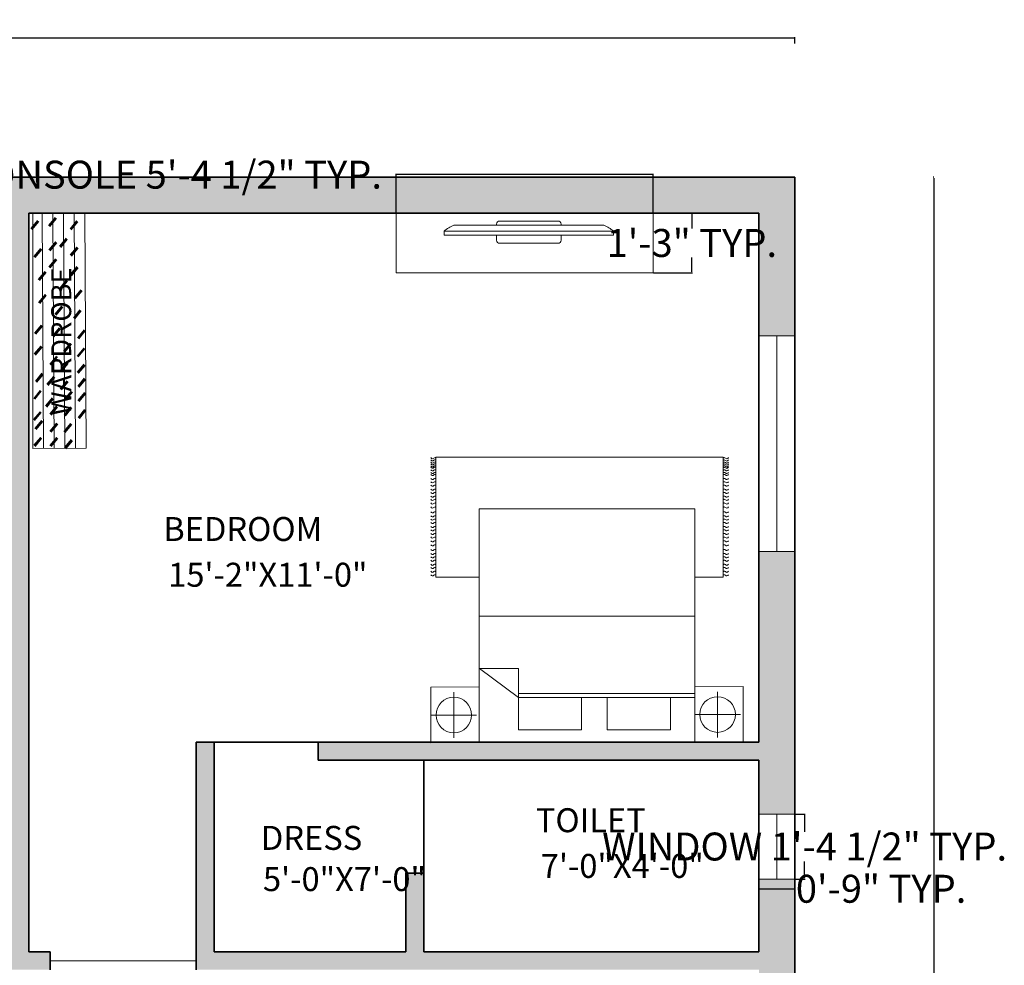
# Model space of a CAD drawing. Units: inches. Extents: x 136 to 672, y -412 to 279.
# Tile 6 of 6: x 409 to 656, y 42 to 279. Entities that reach past the tile are written whole.
import ezdxf

# ---------------------------------------------------------------- set-up
doc = ezdxf.new("R2010")
doc.units = ezdxf.units.IN
doc.header["$MEASUREMENT"] = 0
for name, color, linetype, lineweight in [('A-ANNO-DIMS', 12, 'Continuous', 18), ('A-ANNO-TEXT', 7, 'Continuous', 18), ('A-AREA-IDEN', 7, 'Continuous', 18), ('A-DOOR', 4, 'Continuous', 18), ('A-EQPM', 8, 'Continuous', 18), ('A-FLOR-CASE', 252, 'Continuous', 18), ('A-FLOR-CASE-PATT', 9, 'Continuous', 9), ('A-WALL-PATT', 244, 'Continuous', 9), ('furniture', 252, 'Continuous', 18), ('walls', 253, 'Continuous', 35), ('windows', 171, 'Continuous', 18)]:
    doc.layers.add(name, color=color, linetype=linetype, lineweight=lineweight)
doc.styles.get("Standard").update_dxf_attribs({"font": 'arial.ttf'})
doc.dimstyles.get("Standard").update_dxf_attribs({"dimtxt": 7, "dimasz": 0.18, "dimexe": 0.18, "dimexo": 0.0625, "dimgap": 0.09, "dimtad": 0, "dimtih": 1, "dimtoh": 1, "dimzin": 0, "dimdsep": 46, "dimlunit": 3, "dimtxsty": 'Standard', "dimcen": 0.09, "dimadec": 0, "dimazin": 0, "dimtfac": 1, "dimtofl": 0, "dimtmove": 0, "dimatfit": 3, "dimfxl": 1, "dimtolj": 1, "dimtzin": 0, "dimarcsym": 0})

# ---------------------------------------------------------------- blocks, each defined once
blk = doc.blocks.new('CARPET')
at = {"layer": 'furniture'}
for p, q in [((-51.53, -98.11), (-51.53, -55.12)), ((-51.53, -55.12), (-41.27, -55.12)), ((36, -55.12), (51.55, -55.12)), ((51.55, -55.12), (51.55, -98.11)), ((51.55, -98.11), (-51.53, -98.11))]:
    blk.add_line(p, q, dxfattribs=at)
for points, knots in [([(-53.37, -55.99), (-53.22, -55.8), (-52.9, -55.41), (-52.34, -55.8), (-51.89, -56.08), (-51.65, -55.91), (-51.53, -55.83)], [0, 0, 0, 0, 0.653278, 1.290138, 1.740457, 2.114451, 2.114451, 2.114451, 2.114451]), ([(53.37, -55.99), (53.22, -55.8), (52.9, -55.41), (52.34, -55.8), (51.89, -56.08), (51.65, -55.91), (51.53, -55.83)], [0, 0, 0, 0, 0.653278, 1.290138, 1.740457, 2.114451, 2.114451, 2.114451, 2.114451]), ([(-53.37, -57.26), (-53.22, -57.07), (-52.9, -56.67), (-52.34, -57.07), (-51.89, -57.35), (-51.65, -57.17), (-51.53, -57.1)], [0, 0, 0, 0, 0.653278, 1.290138, 1.740457, 2.114451, 2.114451, 2.114451, 2.114451]), ([(-53.37, -58.59), (-53.22, -58.4), (-52.9, -58.01), (-52.34, -58.4), (-51.89, -58.68), (-51.65, -58.5), (-51.53, -58.43)], [0, 0, 0, 0, 0.653278, 1.290138, 1.740457, 2.114451, 2.114451, 2.114451, 2.114451]), ([(-53.37, -59.78), (-53.22, -59.58), (-52.9, -59.19), (-52.34, -59.58), (-51.89, -59.86), (-51.65, -59.69), (-51.53, -59.61)], [0, 0, 0, 0, 0.653278, 1.290138, 1.740457, 2.114451, 2.114451, 2.114451, 2.114451]), ([(53.37, -57.26), (53.22, -57.07), (52.9, -56.67), (52.34, -57.07), (51.89, -57.35), (51.65, -57.17), (51.53, -57.1)], [0, 0, 0, 0, 0.653278, 1.290138, 1.740457, 2.114451, 2.114451, 2.114451, 2.114451]), ([(53.37, -58.59), (53.22, -58.4), (52.9, -58.01), (52.34, -58.4), (51.89, -58.68), (51.65, -58.5), (51.53, -58.43)], [0, 0, 0, 0, 0.653278, 1.290138, 1.740457, 2.114451, 2.114451, 2.114451, 2.114451]), ([(53.37, -59.78), (53.22, -59.58), (52.9, -59.19), (52.34, -59.58), (51.89, -59.86), (51.65, -59.69), (51.53, -59.61)], [0, 0, 0, 0, 0.653278, 1.290138, 1.740457, 2.114451, 2.114451, 2.114451, 2.114451]), ([(-53.37, -61.22), (-53.22, -61.02), (-52.9, -60.63), (-52.34, -61.02), (-51.89, -61.3), (-51.65, -61.13), (-51.53, -61.05)], [0, 0, 0, 0, 0.653278, 1.290138, 1.740457, 2.114451, 2.114451, 2.114451, 2.114451]), ([(-53.37, -62.44), (-53.22, -62.25), (-52.9, -61.86), (-52.34, -62.25), (-51.89, -62.53), (-51.65, -62.36), (-51.53, -62.28)], [0, 0, 0, 0, 0.653278, 1.290138, 1.740457, 2.114451, 2.114451, 2.114451, 2.114451]), ([(-53.37, -63.63), (-53.22, -63.43), (-52.9, -63.04), (-52.34, -63.43), (-51.89, -63.72), (-51.65, -63.54), (-51.53, -63.46)], [0, 0, 0, 0, 0.653278, 1.290138, 1.740457, 2.114451, 2.114451, 2.114451, 2.114451]), ([(53.37, -61.22), (53.22, -61.02), (52.9, -60.63), (52.34, -61.02), (51.89, -61.3), (51.65, -61.13), (51.53, -61.05)], [0, 0, 0, 0, 0.653278, 1.290138, 1.740457, 2.114451, 2.114451, 2.114451, 2.114451]), ([(53.37, -62.44), (53.22, -62.25), (52.9, -61.86), (52.34, -62.25), (51.89, -62.53), (51.65, -62.36), (51.53, -62.28)], [0, 0, 0, 0, 0.653278, 1.290138, 1.740457, 2.114451, 2.114451, 2.114451, 2.114451]), ([(53.37, -63.63), (53.22, -63.43), (52.9, -63.04), (52.34, -63.43), (51.89, -63.72), (51.65, -63.54), (51.53, -63.46)], [0, 0, 0, 0, 0.653278, 1.290138, 1.740457, 2.114451, 2.114451, 2.114451, 2.114451]), ([(-53.37, -65.07), (-53.22, -64.87), (-52.9, -64.48), (-52.34, -64.87), (-51.89, -65.15), (-51.65, -64.98), (-51.53, -64.9)], [0, 0, 0, 0, 0.653278, 1.290138, 1.740457, 2.114451, 2.114451, 2.114451, 2.114451]), ([(-53.37, -66.76), (-53.22, -66.56), (-52.9, -66.17), (-52.34, -66.56), (-51.89, -66.84), (-51.65, -66.67), (-51.53, -66.59)], [0, 0, 0, 0, 0.653278, 1.290138, 1.740457, 2.114451, 2.114451, 2.114451, 2.114451]), ([(53.37, -65.07), (53.22, -64.87), (52.9, -64.48), (52.34, -64.87), (51.89, -65.15), (51.65, -64.98), (51.53, -64.9)], [0, 0, 0, 0, 0.653278, 1.290138, 1.740457, 2.114451, 2.114451, 2.114451, 2.114451]), ([(53.37, -66.76), (53.22, -66.56), (52.9, -66.17), (52.34, -66.56), (51.89, -66.84), (51.65, -66.67), (51.53, -66.59)], [0, 0, 0, 0, 0.653278, 1.290138, 1.740457, 2.114451, 2.114451, 2.114451, 2.114451]), ([(-53.37, -68.2), (-53.22, -68), (-52.9, -67.61), (-52.34, -68), (-51.89, -68.28), (-51.65, -68.11), (-51.53, -68.03)], [0, 0, 0, 0, 0.653278, 1.290138, 1.740457, 2.114451, 2.114451, 2.114451, 2.114451]), ([(-53.37, -69.53), (-53.22, -69.33), (-52.9, -68.94), (-52.34, -69.33), (-51.89, -69.61), (-51.65, -69.44), (-51.53, -69.36)], [0, 0, 0, 0, 0.653278, 1.290138, 1.740457, 2.114451, 2.114451, 2.114451, 2.114451]), ([(-53.37, -70.79), (-53.22, -70.6), (-52.9, -70.21), (-52.34, -70.6), (-51.89, -70.88), (-51.65, -70.7), (-51.53, -70.63)], [0, 0, 0, 0, 0.653278, 1.290138, 1.740457, 2.114451, 2.114451, 2.114451, 2.114451]), ([(53.37, -68.2), (53.22, -68), (52.9, -67.61), (52.34, -68), (51.89, -68.28), (51.65, -68.11), (51.53, -68.03)], [0, 0, 0, 0, 0.653278, 1.290138, 1.740457, 2.114451, 2.114451, 2.114451, 2.114451]), ([(53.37, -69.53), (53.22, -69.33), (52.9, -68.94), (52.34, -69.33), (51.89, -69.61), (51.65, -69.44), (51.53, -69.36)], [0, 0, 0, 0, 0.653278, 1.290138, 1.740457, 2.114451, 2.114451, 2.114451, 2.114451]), ([(53.37, -70.79), (53.22, -70.6), (52.9, -70.21), (52.34, -70.6), (51.89, -70.88), (51.65, -70.7), (51.53, -70.63)], [0, 0, 0, 0, 0.653278, 1.290138, 1.740457, 2.114451, 2.114451, 2.114451, 2.114451]), ([(-53.37, -72.12), (-53.22, -71.93), (-52.9, -71.54), (-52.34, -71.93), (-51.89, -72.21), (-51.65, -72.04), (-51.53, -71.96)], [0, 0, 0, 0, 0.653278, 1.290138, 1.740457, 2.114451, 2.114451, 2.114451, 2.114451]), ([(-53.37, -73.31), (-53.22, -73.11), (-52.9, -72.72), (-52.34, -73.11), (-51.89, -73.4), (-51.65, -73.22), (-51.53, -73.14)], [0, 0, 0, 0, 0.653278, 1.290138, 1.740457, 2.114451, 2.114451, 2.114451, 2.114451]), ([(53.37, -72.12), (53.22, -71.93), (52.9, -71.54), (52.34, -71.93), (51.89, -72.21), (51.65, -72.04), (51.53, -71.96)], [0, 0, 0, 0, 0.653278, 1.290138, 1.740457, 2.114451, 2.114451, 2.114451, 2.114451]), ([(53.37, -73.31), (53.22, -73.11), (52.9, -72.72), (52.34, -73.11), (51.89, -73.4), (51.65, -73.22), (51.53, -73.14)], [0, 0, 0, 0, 0.653278, 1.290138, 1.740457, 2.114451, 2.114451, 2.114451, 2.114451]), ([(-53.37, -74.75), (-53.22, -74.55), (-52.9, -74.16), (-52.34, -74.55), (-51.89, -74.83), (-51.65, -74.66), (-51.53, -74.58)], [0, 0, 0, 0, 0.653278, 1.290138, 1.740457, 2.114451, 2.114451, 2.114451, 2.114451]), ([(-53.37, -75.98), (-53.22, -75.78), (-52.9, -75.39), (-52.34, -75.78), (-51.89, -76.06), (-51.65, -75.89), (-51.53, -75.81)], [0, 0, 0, 0, 0.653278, 1.290138, 1.740457, 2.114451, 2.114451, 2.114451, 2.114451]), ([(-53.37, -77.16), (-53.22, -76.96), (-52.9, -76.57), (-52.34, -76.96), (-51.89, -77.25), (-51.65, -77.07), (-51.53, -76.99)], [0, 0, 0, 0, 0.653278, 1.290138, 1.740457, 2.114451, 2.114451, 2.114451, 2.114451]), ([(53.37, -74.75), (53.22, -74.55), (52.9, -74.16), (52.34, -74.55), (51.89, -74.83), (51.65, -74.66), (51.53, -74.58)], [0, 0, 0, 0, 0.653278, 1.290138, 1.740457, 2.114451, 2.114451, 2.114451, 2.114451]), ([(53.37, -75.98), (53.22, -75.78), (52.9, -75.39), (52.34, -75.78), (51.89, -76.06), (51.65, -75.89), (51.53, -75.81)], [0, 0, 0, 0, 0.653278, 1.290138, 1.740457, 2.114451, 2.114451, 2.114451, 2.114451]), ([(53.37, -77.16), (53.22, -76.96), (52.9, -76.57), (52.34, -76.96), (51.89, -77.25), (51.65, -77.07), (51.53, -76.99)], [0, 0, 0, 0, 0.653278, 1.290138, 1.740457, 2.114451, 2.114451, 2.114451, 2.114451]), ([(-53.37, -78.6), (-53.22, -78.4), (-52.9, -78.01), (-52.34, -78.4), (-51.89, -78.68), (-51.65, -78.51), (-51.53, -78.43)], [0, 0, 0, 0, 0.653278, 1.290138, 1.740457, 2.114451, 2.114451, 2.114451, 2.114451]), ([(-53.37, -80.29), (-53.22, -80.09), (-52.9, -79.7), (-52.34, -80.09), (-51.89, -80.37), (-51.65, -80.2), (-51.53, -80.12)], [0, 0, 0, 0, 0.653278, 1.290138, 1.740457, 2.114451, 2.114451, 2.114451, 2.114451]), ([(53.37, -78.6), (53.22, -78.4), (52.9, -78.01), (52.34, -78.4), (51.89, -78.68), (51.65, -78.51), (51.53, -78.43)], [0, 0, 0, 0, 0.653278, 1.290138, 1.740457, 2.114451, 2.114451, 2.114451, 2.114451]), ([(53.37, -80.29), (53.22, -80.09), (52.9, -79.7), (52.34, -80.09), (51.89, -80.37), (51.65, -80.2), (51.53, -80.12)], [0, 0, 0, 0, 0.653278, 1.290138, 1.740457, 2.114451, 2.114451, 2.114451, 2.114451]), ([(-53.37, -81.73), (-53.22, -81.53), (-52.9, -81.14), (-52.34, -81.53), (-51.89, -81.81), (-51.65, -81.64), (-51.53, -81.56)], [0, 0, 0, 0, 0.653278, 1.290138, 1.740457, 2.114451, 2.114451, 2.114451, 2.114451]), ([(-53.37, -83.06), (-53.22, -82.86), (-52.9, -82.47), (-52.34, -82.86), (-51.89, -83.14), (-51.65, -82.97), (-51.53, -82.89)], [0, 0, 0, 0, 0.653278, 1.290138, 1.740457, 2.114451, 2.114451, 2.114451, 2.114451]), ([(-53.37, -84.18), (-53.22, -83.99), (-52.9, -83.6), (-52.34, -83.99), (-51.89, -84.27), (-51.65, -84.09), (-51.53, -84.02)], [0, 0, 0, 0, 0.653278, 1.290138, 1.740457, 2.114451, 2.114451, 2.114451, 2.114451]), ([(53.37, -81.73), (53.22, -81.53), (52.9, -81.14), (52.34, -81.53), (51.89, -81.81), (51.65, -81.64), (51.53, -81.56)], [0, 0, 0, 0, 0.653278, 1.290138, 1.740457, 2.114451, 2.114451, 2.114451, 2.114451]), ([(53.37, -83.06), (53.22, -82.86), (52.9, -82.47), (52.34, -82.86), (51.89, -83.14), (51.65, -82.97), (51.53, -82.89)], [0, 0, 0, 0, 0.653278, 1.290138, 1.740457, 2.114451, 2.114451, 2.114451, 2.114451]), ([(53.37, -84.18), (53.22, -83.99), (52.9, -83.6), (52.34, -83.99), (51.89, -84.27), (51.65, -84.09), (51.53, -84.02)], [0, 0, 0, 0, 0.653278, 1.290138, 1.740457, 2.114451, 2.114451, 2.114451, 2.114451]), ([(-53.37, -85.51), (-53.22, -85.32), (-52.9, -84.93), (-52.34, -85.32), (-51.89, -85.6), (-51.65, -85.42), (-51.53, -85.35)], [0, 0, 0, 0, 0.653278, 1.290138, 1.740457, 2.114451, 2.114451, 2.114451, 2.114451]), ([(-53.37, -86.7), (-53.22, -86.5), (-52.9, -86.11), (-52.34, -86.5), (-51.89, -86.78), (-51.65, -86.61), (-51.53, -86.53)], [0, 0, 0, 0, 0.653278, 1.290138, 1.740457, 2.114451, 2.114451, 2.114451, 2.114451]), ([(-53.37, -88.14), (-53.22, -87.94), (-52.9, -87.55), (-52.34, -87.94), (-51.89, -88.22), (-51.65, -88.05), (-51.53, -87.97)], [0, 0, 0, 0, 0.653278, 1.290138, 1.740457, 2.114451, 2.114451, 2.114451, 2.114451]), ([(53.37, -85.51), (53.22, -85.32), (52.9, -84.93), (52.34, -85.32), (51.89, -85.6), (51.65, -85.42), (51.53, -85.35)], [0, 0, 0, 0, 0.653278, 1.290138, 1.740457, 2.114451, 2.114451, 2.114451, 2.114451]), ([(53.37, -86.7), (53.22, -86.5), (52.9, -86.11), (52.34, -86.5), (51.89, -86.78), (51.65, -86.61), (51.53, -86.53)], [0, 0, 0, 0, 0.653278, 1.290138, 1.740457, 2.114451, 2.114451, 2.114451, 2.114451]), ([(53.37, -88.14), (53.22, -87.94), (52.9, -87.55), (52.34, -87.94), (51.89, -88.22), (51.65, -88.05), (51.53, -87.97)], [0, 0, 0, 0, 0.653278, 1.290138, 1.740457, 2.114451, 2.114451, 2.114451, 2.114451]), ([(-53.37, -89.36), (-53.22, -89.17), (-52.9, -88.78), (-52.34, -89.17), (-51.89, -89.45), (-51.65, -89.28), (-51.53, -89.2)], [0, 0, 0, 0, 0.653278, 1.290138, 1.740457, 2.114451, 2.114451, 2.114451, 2.114451]), ([(-53.37, -90.55), (-53.22, -90.35), (-52.9, -89.96), (-52.34, -90.35), (-51.89, -90.64), (-51.65, -90.46), (-51.53, -90.38)], [0, 0, 0, 0, 0.653278, 1.290138, 1.740457, 2.114451, 2.114451, 2.114451, 2.114451]), ([(-53.37, -91.99), (-53.22, -91.79), (-52.9, -91.4), (-52.34, -91.79), (-51.89, -92.07), (-51.65, -91.9), (-51.53, -91.82)], [0, 0, 0, 0, 0.653278, 1.290138, 1.740457, 2.114451, 2.114451, 2.114451, 2.114451]), ([(53.37, -89.36), (53.22, -89.17), (52.9, -88.78), (52.34, -89.17), (51.89, -89.45), (51.65, -89.28), (51.53, -89.2)], [0, 0, 0, 0, 0.653278, 1.290138, 1.740457, 2.114451, 2.114451, 2.114451, 2.114451]), ([(53.37, -90.55), (53.22, -90.35), (52.9, -89.96), (52.34, -90.35), (51.9, -90.63), (51.66, -90.47), (51.55, -90.4)], [0, 0, 0, 0, 0.653278, 1.290138, 1.740457, 2.0926, 2.0926, 2.0926, 2.0926]), ([(53.37, -91.99), (53.22, -91.79), (52.9, -91.4), (52.34, -91.79), (51.9, -92.07), (51.66, -91.91), (51.55, -91.83)], [0, 0, 0, 0, 0.653278, 1.290138, 1.740457, 2.0926, 2.0926, 2.0926, 2.0926]), ([(-53.37, -92.69), (-53.22, -92.48), (-52.9, -92.08), (-52.35, -92.49), (-51.89, -92.77), (-51.65, -92.6), (-51.53, -92.52)], [0, 0, 0, 0, 0.663904, 1.307406, 1.757725, 2.131719, 2.131719, 2.131719, 2.131719]), ([(-53.37, -93.61), (-53.22, -93.42), (-52.9, -93.03), (-52.34, -93.42), (-51.89, -93.7), (-51.65, -93.52), (-51.53, -93.45)], [0, 0, 0, 0, 0.653278, 1.290138, 1.740457, 2.114451, 2.114451, 2.114451, 2.114451]), ([(-53.37, -94.55), (-53.22, -94.35), (-52.9, -93.96), (-52.34, -94.35), (-51.89, -94.63), (-51.65, -94.46), (-51.53, -94.38)], [0, 0, 0, 0, 0.653278, 1.290138, 1.740457, 2.114451, 2.114451, 2.114451, 2.114451]), ([(-53.37, -95.05), (-53.22, -94.85), (-52.9, -94.46), (-52.34, -94.85), (-51.89, -95.14), (-51.65, -94.96), (-51.53, -94.88)], [0, 0, 0, 0, 0.653278, 1.290138, 1.740457, 2.114451, 2.114451, 2.114451, 2.114451]), ([(-53.37, -95.73), (-53.22, -95.54), (-52.9, -95.15), (-52.34, -95.54), (-51.89, -95.82), (-51.65, -95.65), (-51.53, -95.57)], [0, 0, 0, 0, 0.653278, 1.290138, 1.740457, 2.114451, 2.114451, 2.114451, 2.114451]), ([(53.37, -95.78), (53.22, -95.58), (52.9, -95.19), (52.34, -95.58), (51.89, -95.86), (51.65, -95.69), (51.53, -95.61)], [0, 0, 0, 0, 0.653278, 1.290138, 1.740457, 2.114451, 2.114451, 2.114451, 2.114451]), ([(53.37, -92.69), (53.22, -92.49), (52.9, -92.09), (52.34, -92.49), (51.9, -92.77), (51.66, -92.61), (51.55, -92.53)], [0, 0, 0, 0, 0.656792, 1.295826, 1.746145, 2.098292, 2.098292, 2.098292, 2.098292]), ([(53.37, -93.66), (53.22, -93.46), (52.9, -93.07), (52.34, -93.46), (51.9, -93.74), (51.66, -93.58), (51.55, -93.5)], [0, 0, 0, 0, 0.653278, 1.290138, 1.740457, 2.0926, 2.0926, 2.0926, 2.0926]), ([(53.37, -94.59), (53.22, -94.4), (52.9, -94.01), (52.34, -94.4), (51.9, -94.68), (51.66, -94.51), (51.55, -94.44)], [0, 0, 0, 0, 0.653278, 1.290138, 1.740457, 2.0926, 2.0926, 2.0926, 2.0926]), ([(53.37, -95.1), (53.22, -94.9), (52.9, -94.51), (52.34, -94.9), (51.9, -95.18), (51.66, -95.02), (51.55, -94.94)], [0, 0, 0, 0, 0.653278, 1.290138, 1.740457, 2.0926, 2.0926, 2.0926, 2.0926]), ([(-53.37, -96.38), (-53.22, -96.18), (-52.9, -95.79), (-52.34, -96.18), (-51.89, -96.47), (-51.65, -96.29), (-51.53, -96.21)], [0, 0, 0, 0, 0.653278, 1.290138, 1.740457, 2.114451, 2.114451, 2.114451, 2.114451]), ([(-53.37, -97.17), (-53.22, -96.98), (-52.9, -96.59), (-52.34, -96.98), (-51.89, -97.26), (-51.65, -97.08), (-51.53, -97.01)], [0, 0, 0, 0, 0.653278, 1.290138, 1.740457, 2.114451, 2.114451, 2.114451, 2.114451]), ([(-53.37, -97.99), (-53.22, -97.79), (-52.9, -97.4), (-52.34, -97.79), (-51.89, -98.08), (-51.65, -97.9), (-51.53, -97.82)], [0, 0, 0, 0, 0.653278, 1.290138, 1.740457, 2.114451, 2.114451, 2.114451, 2.114451]), ([(53.37, -96.43), (53.22, -96.23), (52.9, -95.84), (52.34, -96.23), (51.89, -96.51), (51.65, -96.34), (51.53, -96.26)], [0, 0, 0, 0, 0.653278, 1.290138, 1.740457, 2.114451, 2.114451, 2.114451, 2.114451]), ([(53.37, -97.22), (53.22, -97.02), (52.9, -96.63), (52.34, -97.02), (51.89, -97.3), (51.65, -97.13), (51.53, -97.05)], [0, 0, 0, 0, 0.653278, 1.290138, 1.740457, 2.114451, 2.114451, 2.114451, 2.114451]), ([(53.37, -97.99), (53.22, -97.79), (52.9, -97.4), (52.34, -97.79), (51.89, -98.08), (51.65, -97.9), (51.53, -97.82)], [0, 0, 0, 0, 0.653278, 1.290138, 1.740457, 2.114451, 2.114451, 2.114451, 2.114451])]:
    blk.add_open_spline(points, degree=3, knots=knots, dxfattribs=at)
blk = doc.blocks.new('A$C58D270C6')
at = {"layer": 'furniture'}
for p, q in [((9.09, 124.13), (9.09, 108.87)), ((1.46, 116.5), (16.73, 116.5)), ((14.97, 94.84), (24.62, 107.92)), ((24.62, 94.93), (24.62, 107.92)), ((42.08, 108), (42.08, 36)), ((14.97, 94.93), (24.62, 94.93)), ((14.97, 94.84), (14.97, 36)), ((16.22, 94.93), (16.22, 36)), ((9.25, 36), (9.25, 20.74)), ((1.62, 28.37), (16.88, 28.37))]:
    blk.add_line(p, q, dxfattribs=at)
for points in [[(18.5, 108), (18.34, 124.13), (-0.16, 124.13), (0, 108)], [(0, 108), (77.91, 108), (77.91, 36), (0, 36)], [(4.09, 94.93), (14.97, 94.93), (14.97, 73.83), (4.09, 73.83)], [(4.09, 65.23), (14.97, 65.23), (14.97, 44.13), (4.09, 44.13)], [(18.65, 19.87), (18.5, 36), (0, 36), (0.16, 19.87)]]:
    blk.add_lwpolyline(points, close=True, dxfattribs=at)
for centre in [(9.09, 116.5), (9.25, 28.37)]:
    blk.add_circle(centre, 5.95, dxfattribs=at)
at = {"layer": 'furniture', "xscale": 0.9312884925094044, "yscale": 0.9312884925094044, "zscale": 0.9312884925094044, "rotation": 90}
blk.add_blockref('CARPET', (3.79, 74.47), dxfattribs=at)
blk = doc.blocks.new('PLASMA-LARGE')
at = {"layer": 'furniture'}
for p, q in [((-7.26, 0), (7.26, 0)), ((-18.61, -1), (18.61, -1)), ((-8, -1), (-8, -0.74)), ((8, -1), (8, -0.74)), ((-21, -2.5), (21, -2.5)), ((-21, -2.5), (-21, -3.5)), ((-21, -3.5), (21, -3.5)), ((-8, -3.5), (-8, -4.76)), ((8, -3.5), (8, -4.76)), ((21, -2.5), (21, -3.5)), ((-7.26, -5.5), (7.26, -5.5))]:
    blk.add_line(p, q, dxfattribs=at)
for centre, radius, start, end in [((-7.26, -0.74), 0.744, 90, 180), ((7.26, -0.74), 0.744, 0, 90), ((-13.97, -11.05), 11.07, 114.7602, 129.4175), ((13.97, -11.05), 11.07, 50.5825, 65.2398), ((-7.26, -4.76), 0.744, 180, 270), ((7.26, -4.76), 0.744, 270, 0)]:
    blk.add_arc(centre, radius, start, end, dxfattribs=at)
blk = doc.blocks.new('*D18')
at = {"layer": 'A-ANNO-DIMS', "color": 0, "lineweight": -2, "transparency": 16777216}
for p, q in [((183.46, 273.1), (183.46, 274.63)), ((183.64, 274.45), (387.44, 274.45)), ((603.28, 274.45), (399.49, 274.45)), ((603.46, 273.1), (603.46, 274.63))]:
    blk.add_line(p, q, dxfattribs=at)
at = {"layer": 'A-ANNO-DIMS', "color": 0, "transparency": 16777216}
for points in [[(183.64, 274.48), (183.64, 274.42), (183.46, 274.45)], [(603.28, 274.48), (603.28, 274.42), (603.46, 274.45)]]:
    blk.add_solid(points, dxfattribs=at)
at = {"layer": 'Defpoints', "color": 0, "transparency": 16777216}
for p in [(603.46, 274.45), (183.46, 273.04), (603.46, 273.04)]:
    blk.add_point(p, dxfattribs=at)
at = {"layer": 'A-ANNO-DIMS', "color": 0, "transparency": 16777216, "insert": (393.46, 274.45), "char_height": 7, "attachment_point": 5}
blk.add_mtext("\\A1;35'", dxfattribs=at)
blk = doc.blocks.new('*D20')
at = {"layer": 'A-ANNO-DIMS', "color": 0, "lineweight": -2, "transparency": 16777216}
for p, q in [((638.31, 239.56), (638.1, 239.56)), ((638.28, 239.38), (638.28, -56.02)), ((638.28, -358.76), (638.28, -63.35)), ((638.31, -358.94), (638.1, -358.94))]:
    blk.add_line(p, q, dxfattribs=at)
at = {"layer": 'A-ANNO-DIMS', "color": 0, "transparency": 16777216}
for points in [[(638.25, 239.38), (638.31, 239.38), (638.28, 239.56)], [(638.25, -358.76), (638.31, -358.76), (638.28, -358.94)]]:
    blk.add_solid(points, dxfattribs=at)
at = {"layer": 'Defpoints', "color": 0, "transparency": 16777216}
for p in [(638.37, 239.56), (638.28, -358.94), (638.37, -358.94)]:
    blk.add_point(p, dxfattribs=at)
at = {"layer": 'A-ANNO-DIMS', "color": 0, "transparency": 16777216, "insert": (638.28, -59.69), "char_height": 7, "attachment_point": 5}
blk.add_mtext("\\A1;50'", dxfattribs=at)
blk = doc.blocks.new('WIN-54')
for p, q in [((0, 54.05), (9, 54.05)), ((0, 0), (0, 54.05)), ((0, 54.05), (4.5, 54.05)), ((4.5, 54.05), (4.5, 0)), ((9, 54.05), (9, 0)), ((9, 0), (0, 0))]:
    blk.add_line(p, q)
blk = doc.blocks.new('WIN-16')
for p, q in [((0, 16.27), (9, 16.27)), ((0, 0), (0, 16.27)), ((0, 16.27), (4.5, 16.27)), ((4.5, 16.27), (4.5, 0)), ((9, 16.27), (9, 0)), ((9, 0), (0, 0))]:
    blk.add_line(p, q)
blk = doc.blocks.new('CONSOLE-TV')
for p, q in [((0, 0), (0, 64.44)), ((0, 64.44), (14.9, 64.44)), ((14.9, 0), (0, 0))]:
    blk.add_line(p, q)
blk = doc.blocks.new('WARDROBE-FRAME')
for p, q in [((0, 13.37), (58.88, 13.37)), ((0.05, 13.37), (0.13, 0)), ((58.95, 0.34), (58.88, 13.71)), ((0.02, 10.69), (58.89, 11.04)), ((0.03, 8.02), (58.91, 8.36)), ((0.05, 5.35), (58.92, 5.69)), ((0.06, 2.67), (58.94, 3.02)), ((0.08, 0), (58.95, 0.34))]:
    blk.add_line(p, q)
blk = doc.blocks.new('*D31')
at = {"layer": 'A-ANNO-DIMS', "color": 0, "lineweight": -2, "transparency": 16777216}
for p, q in [((503.53, 240.23), (503.35, 240.23)), ((503.53, 230.63), (503.53, 240.41)), ((567.79, 240.23), (503.71, 240.23)), ((567.97, 230.63), (567.97, 240.41))]:
    blk.add_line(p, q, dxfattribs=at)
at = {"layer": 'A-ANNO-DIMS', "color": 0, "transparency": 16777216}
for points in [[(503.71, 240.26), (503.71, 240.2), (503.53, 240.23)], [(567.79, 240.26), (567.79, 240.2), (567.97, 240.23)]]:
    blk.add_solid(points, dxfattribs=at)
at = {"layer": 'Defpoints', "color": 0, "transparency": 16777216}
for p in [(503.53, 240.23), (503.53, 230.56), (567.97, 230.56)]:
    blk.add_point(p, dxfattribs=at)
at = {"layer": 'A-ANNO-DIMS', "color": 0, "transparency": 16777216, "insert": (440.81, 240.23), "char_height": 7, "attachment_point": 5}
blk.add_mtext('\\A1;TV CONSOLE 5\'-4 1/2" TYP.', dxfattribs=at)
blk = doc.blocks.new('*D32')
at = {"layer": 'A-ANNO-DIMS', "color": 0, "lineweight": -2, "transparency": 16777216}
for p, q in [((568.04, 230.56), (577.82, 230.56)), ((577.64, 230.38), (577.64, 226.78)), ((577.64, 215.85), (577.64, 219.45)), ((568.04, 215.67), (577.82, 215.67))]:
    blk.add_line(p, q, dxfattribs=at)
at = {"layer": 'A-ANNO-DIMS', "color": 0, "transparency": 16777216}
for points in [[(577.61, 230.38), (577.67, 230.38), (577.64, 230.56)], [(577.61, 215.85), (577.67, 215.85), (577.64, 215.67)]]:
    blk.add_solid(points, dxfattribs=at)
at = {"layer": 'Defpoints', "color": 0, "transparency": 16777216}
for p in [(567.97, 230.56), (577.64, 230.56), (567.97, 215.67)]:
    blk.add_point(p, dxfattribs=at)
at = {"layer": 'A-ANNO-DIMS', "color": 0, "transparency": 16777216, "insert": (577.64, 223.12), "char_height": 7, "attachment_point": 5}
blk.add_mtext('\\A1;1\'-3" TYP.', dxfattribs=at)
blk = doc.blocks.new('*D51')
at = {"layer": 'A-ANNO-DIMS', "color": 0, "lineweight": -2, "transparency": 16777216}
for p, q in [((603.53, 80.07), (606.08, 80.07)), ((605.9, 79.89), (605.9, 75.65)), ((605.9, 63.98), (605.9, 68.23)), ((603.53, 63.8), (606.08, 63.8))]:
    blk.add_line(p, q, dxfattribs=at)
at = {"layer": 'A-ANNO-DIMS', "color": 0, "transparency": 16777216}
for points in [[(605.87, 79.89), (605.93, 79.89), (605.9, 80.07)], [(605.87, 63.98), (605.93, 63.98), (605.9, 63.8)]]:
    blk.add_solid(points, dxfattribs=at)
at = {"layer": 'Defpoints', "color": 0, "transparency": 16777216}
for p in [(603.46, 80.07), (605.9, 80.07), (603.46, 63.8)]:
    blk.add_point(p, dxfattribs=at)
at = {"layer": 'A-ANNO-DIMS', "color": 0, "transparency": 16777216, "insert": (605.9, 71.94), "char_height": 7, "attachment_point": 5}
blk.add_mtext('\\A1;WINDOW 1\'-4 1/2" TYP.', dxfattribs=at)
blk = doc.blocks.new('*D52')
at = {"layer": 'A-ANNO-DIMS', "color": 0, "lineweight": -2, "transparency": 16777216}
for p, q in [((594.46, 63.74), (594.46, 61.18)), ((603.46, 63.74), (603.46, 61.18)), ((594.64, 61.36), (603.28, 61.36)), ((603.46, 61.36), (603.64, 61.36))]:
    blk.add_line(p, q, dxfattribs=at)
at = {"layer": 'A-ANNO-DIMS', "color": 0, "transparency": 16777216}
for points in [[(594.64, 61.39), (594.64, 61.33), (594.46, 61.36)], [(603.28, 61.39), (603.28, 61.33), (603.46, 61.36)]]:
    blk.add_solid(points, dxfattribs=at)
at = {"layer": 'Defpoints', "color": 0, "transparency": 16777216}
for p in [(594.46, 63.8), (603.46, 63.8), (603.46, 61.36)]:
    blk.add_point(p, dxfattribs=at)
at = {"layer": 'A-ANNO-DIMS', "color": 0, "transparency": 16777216, "insert": (625.07, 61.36), "char_height": 7, "attachment_point": 5}
blk.add_mtext('\\A1;0\'-9" TYP.', dxfattribs=at)

msp = doc.modelspace()

# ---------------------------------------------------------------- hatches: boundary and pattern name
at = {"layer": 'A-FLOR-CASE-PATT'}
h = msp.add_hatch(dxfattribs=at)
h.set_pattern_fill('ANSI31', color=256, scale=0.847566, angle=5.46701, style=0)
h.paths.add_polyline_path([(418.117, 229.497), (416.469, 227.5), (416.801, 227.226), (418.449, 229.223)])
h = msp.add_hatch(dxfattribs=at)
h.set_pattern_fill('ANSI31', color=256, scale=0.8476654, angle=5.467005, style=0)
h.paths.add_polyline_path([(413.668, 228.734), (412.02, 226.737), (412.351, 226.463), (413.999, 228.46)])
h = msp.add_hatch(dxfattribs=at)
h.set_pattern_fill('ANSI31', color=256, scale=0.8474634, angle=5.467005, style=0)
h.paths.add_polyline_path([(423.469, 228.692), (421.82, 226.695), (422.152, 226.421), (423.8, 228.418)])
h = msp.add_hatch(dxfattribs=at)
h.set_pattern_fill('ANSI31', color=256, scale=0.847412, angle=5.46701, style=0)
h.paths.add_polyline_path([(418.153, 223.433), (416.505, 221.436), (416.836, 221.162), (418.484, 223.159)])
h = msp.add_hatch(dxfattribs=at)
h.set_pattern_fill('ANSI31', color=256, scale=0.8475639, angle=5.467005, style=0)
h.paths.add_polyline_path([(420.821, 224.285), (419.173, 222.288), (419.505, 222.014), (421.153, 224.011)])
h = msp.add_hatch(dxfattribs=at)
h.set_pattern_fill('ANSI31', color=256, scale=0.8473947, angle=5.467005, style=0)
h.paths.add_polyline_path([(423.507, 222.105), (421.859, 220.108), (422.191, 219.834), (423.839, 221.831)])
h = msp.add_hatch(dxfattribs=at)
h.set_pattern_fill('ANSI31', color=256, scale=0.8473185, angle=5.467005, style=0)
h.paths.add_polyline_path([(414.392, 221.736), (412.744, 219.739), (413.076, 219.466), (414.724, 221.462)])
h = msp.add_hatch(dxfattribs=at)
h.set_pattern_fill('ANSI31', color=256, scale=0.847383, angle=5.46701, style=0)
h.paths.add_polyline_path([(418.178, 219.146), (416.53, 217.149), (416.862, 216.876), (418.51, 218.873)])
h = msp.add_hatch(dxfattribs=at)
h.set_pattern_fill('ANSI31', color=256, scale=0.847746, angle=5.46701, style=0)
h.paths.add_polyline_path([(423.536, 217.191), (421.888, 215.194), (422.22, 214.921), (423.868, 216.917)])
h = msp.add_hatch(dxfattribs=at)
h.set_pattern_fill('ANSI31', color=256, scale=0.8476829, angle=5.467005, style=0)
h.paths.add_polyline_path([(415.523, 215.994), (413.875, 213.997), (414.207, 213.724), (415.855, 215.72)])
h = msp.add_hatch(dxfattribs=at)
h.set_pattern_fill('ANSI31', color=256, scale=0.8476873, angle=5.467005, style=0)
h.paths.add_polyline_path([(420.882, 213.83), (419.234, 211.833), (419.566, 211.559), (421.214, 213.556)])
h = msp.add_hatch(dxfattribs=at)
h.set_pattern_fill('ANSI31', color=256, scale=0.8475809, angle=5.467005, style=0)
h.paths.add_polyline_path([(415.557, 210.244), (413.909, 208.247), (414.24, 207.973), (415.888, 209.97)])
h = msp.add_hatch(dxfattribs=at)
h.set_pattern_fill('ANSI31', color=256, scale=0.8473222, angle=5.467005, style=0)
h.paths.add_polyline_path([(424.532, 211.391), (422.884, 209.394), (423.215, 209.12), (424.863, 211.117)])
h = msp.add_hatch(dxfattribs=at)
h.set_pattern_fill('ANSI31', color=256, scale=0.8474212, angle=5.467005, style=0)
h.paths.add_polyline_path([(419.687, 207.316), (418.039, 205.319), (418.371, 205.046), (420.019, 207.042)])
h = msp.add_hatch(dxfattribs=at)
h.set_pattern_fill('ANSI31', color=256, scale=0.8476181, angle=5.467005, style=0)
h.paths.add_polyline_path([(424.316, 206.362), (422.668, 204.366), (422.999, 204.092), (424.647, 206.089)])
h = msp.add_hatch(dxfattribs=at)
h.set_pattern_fill('ANSI31', color=256, scale=0.8477215, angle=5.467005, style=0)
h.paths.add_polyline_path([(414.602, 202.545), (412.954, 200.548), (413.285, 200.275), (414.933, 202.272)])
h = msp.add_hatch(dxfattribs=at)
h.set_pattern_fill('ANSI31', color=256, scale=0.8476278, angle=5.467005, style=0)
h.paths.add_polyline_path([(419.106, 201.877), (417.457, 199.88), (417.789, 199.606), (419.437, 201.603)])
h = msp.add_hatch(dxfattribs=at)
h.set_pattern_fill('ANSI31', color=256, scale=0.8473198, angle=5.467005, style=0)
h.paths.add_polyline_path([(425.327, 201.373), (423.679, 199.376), (424.01, 199.102), (425.658, 201.099)])
h = msp.add_hatch(dxfattribs=at)
h.set_pattern_fill('ANSI31', color=256, scale=0.8475636, angle=5.467005, style=0)
h.paths.add_polyline_path([(421.828, 198.042), (420.18, 196.045), (420.512, 195.771), (422.16, 197.768)])
h = msp.add_hatch(dxfattribs=at)
h.set_pattern_fill('ANSI31', color=256, scale=0.8476097, angle=5.467005, style=0)
h.paths.add_polyline_path([(414.51, 197.313), (412.861, 195.316), (413.193, 195.043), (414.841, 197.04)])
h = msp.add_hatch(dxfattribs=at)
h.set_pattern_fill('ANSI31', color=256, scale=0.8473692, angle=5.467005, style=0)
h.paths.add_polyline_path([(425.275, 196.798), (423.627, 194.802), (423.877, 194.595), (425.525, 196.592)])
h = msp.add_hatch(dxfattribs=at)
h.set_pattern_fill('ANSI31', color=256, scale=0.847447, angle=5.46701, style=0)
h.paths.add_polyline_path([(418.402, 194.766), (416.754, 192.769), (417.004, 192.563), (418.652, 194.56)])
h = msp.add_hatch(dxfattribs=at)
h.set_pattern_fill('ANSI31', color=256, scale=0.8476638, angle=5.467005, style=0)
h.paths.add_polyline_path([(421.003, 193.177), (419.355, 191.18), (419.687, 190.906), (421.335, 192.903)])
h = msp.add_hatch(dxfattribs=at)
h.set_pattern_fill('ANSI31', color=256, scale=0.847498, angle=5.46701, style=0)
h.paths.add_polyline_path([(425.263, 192.741), (423.615, 190.744), (423.946, 190.471), (425.594, 192.467)])
h = msp.add_hatch(dxfattribs=at)
h.set_pattern_fill('ANSI31', color=256, scale=0.8476678, angle=5.467005, style=0)
h.paths.add_polyline_path([(414.795, 190.48), (413.147, 188.483), (413.479, 188.21), (415.127, 190.207)])
h = msp.add_hatch(dxfattribs=at)
h.set_pattern_fill('ANSI31', color=256, scale=0.8474445, angle=5.467005, style=0)
h.paths.add_polyline_path([(417.663, 189.711), (416.015, 187.714), (416.347, 187.441), (417.995, 189.437)])
h = msp.add_hatch(dxfattribs=at)
h.set_pattern_fill('ANSI31', color=256, scale=0.8475369, angle=5.467005, style=0)
h.paths.add_polyline_path([(421.03, 188.597), (419.382, 186.6), (419.714, 186.326), (421.362, 188.323)])
h = msp.add_hatch(dxfattribs=at)
h.set_pattern_fill('ANSI31', color=256, scale=0.8475593, angle=5.467005, style=0)
h.paths.add_polyline_path([(425.408, 189.232), (423.76, 187.235), (424.092, 186.961), (425.74, 188.958)])
h = msp.add_hatch(dxfattribs=at)
h.set_pattern_fill('ANSI31', color=256, scale=0.847522, angle=5.46701, style=0)
h.paths.add_polyline_path([(414.37, 186.191), (412.722, 184.194), (412.972, 183.988), (414.62, 185.985)])
h = msp.add_hatch(dxfattribs=at)
h.set_pattern_fill('ANSI31', color=256, scale=0.8476648, angle=5.467005, style=0)
h.paths.add_polyline_path([(422.079, 185.99), (420.431, 183.993), (420.763, 183.72), (422.411, 185.716)])
h = msp.add_hatch(dxfattribs=at)
h.set_pattern_fill('ANSI31', color=256, scale=0.8473643, angle=5.467005, style=0)
h.paths.add_polyline_path([(425.429, 185.672), (423.781, 183.675), (424.113, 183.402), (425.761, 185.398)])
h = msp.add_hatch(dxfattribs=at)
h.set_pattern_fill('ANSI31', color=256, scale=0.8474402, angle=5.467005, style=0)
h.paths.add_polyline_path([(417.31, 184.292), (415.662, 182.295), (415.993, 182.021), (417.641, 184.018)])
h = msp.add_hatch(dxfattribs=at)
h.set_pattern_fill('ANSI31', color=256, scale=0.847464, angle=5.46701, style=0)
h.paths.add_polyline_path([(414.349, 180.862), (412.701, 178.865), (412.951, 178.659), (414.599, 180.655)])
h = msp.add_hatch(dxfattribs=at)
h.set_pattern_fill('ANSI31', color=256, scale=0.8473865, angle=5.467005, style=0)
h.paths.add_polyline_path([(418.394, 182.297), (416.746, 180.301), (417.077, 180.027), (418.726, 182.024)])
h = msp.add_hatch(dxfattribs=at)
h.set_pattern_fill('ANSI31', color=256, scale=0.847611, angle=5.46701, style=0)
h.paths.add_polyline_path([(421.98, 182.063), (420.332, 180.066), (420.664, 179.792), (422.312, 181.789)])
h = msp.add_hatch(dxfattribs=at)
h.set_pattern_fill('ANSI31', color=256, scale=0.847377, angle=5.46701, style=0)
h.paths.add_polyline_path([(425.484, 181.407), (423.836, 179.41), (424.168, 179.137), (425.816, 181.133)])
h = msp.add_hatch(dxfattribs=at)
h.set_pattern_fill('ANSI31', color=256, scale=0.8472968, angle=5.467005, style=0)
h.paths.add_polyline_path([(414.689, 178.674), (413.041, 176.677), (413.372, 176.404), (415.02, 178.401)])
h = msp.add_hatch(dxfattribs=at)
h.set_pattern_fill('ANSI31', color=256, scale=0.847381, angle=5.46701, style=0)
h.paths.add_polyline_path([(418.419, 178.003), (416.771, 176.007), (417.103, 175.733), (418.751, 177.73)])
h = msp.add_hatch(dxfattribs=at)
h.set_pattern_fill('ANSI31', color=256, scale=0.8474172, angle=5.467005, style=0)
h.paths.add_polyline_path([(421.931, 177.918), (420.283, 175.921), (420.615, 175.647), (422.263, 177.644)])
h = msp.add_hatch(dxfattribs=at)
h.set_pattern_fill('ANSI31', color=256, scale=0.847437, angle=5.46701, style=0)
h.paths.add_polyline_path([(414.39, 174.431), (412.742, 172.434), (413.074, 172.16), (414.722, 174.157)])
h = msp.add_hatch(dxfattribs=at)
h.set_pattern_fill('ANSI31', color=256, scale=0.8476488, angle=5.467005, style=0)
h.paths.add_polyline_path([(418.44, 174.429), (416.792, 172.432), (417.124, 172.158), (418.772, 174.155)])
h = msp.add_hatch(dxfattribs=at)
h.set_pattern_fill('ANSI31', color=256, scale=0.8476282, angle=5.467005, style=0)
h.paths.add_polyline_path([(422.082, 173.857), (420.434, 171.86), (420.766, 171.586), (422.414, 173.583)])
at = {"layer": 'A-WALL-PATT'}
h = msp.add_hatch(color=256, dxfattribs=at)
h.dxf.hatch_style = 1
h.paths.add_polyline_path([(255.026, 239.565), (183.463, 239.565), (183.463, 125.252), (187.963, 125.252), (192.463, 125.252), (192.463, 230.565), (255.024, 230.565), (255.025, 235.065)])
h.paths.add_polyline_path([(369.355, 239.565), (332.259, 239.565), (332.259, 230.565), (342.463, 230.565), (342.463, 104.521), (346.963, 104.521), (346.963, 230.565), (369.355, 230.565), (369.355, 235.065)])
h.paths.add_polyline_path([(603.463, 239.565), (385.627, 239.565), (385.627, 230.565), (406.963, 230.565), (406.963, 134.565), (371.802, 134.565), (371.802, 130.065), (406.963, 130.065), (406.963, 45.565), (346.963, 45.565), (346.963, 69.395), (342.463, 69.395), (342.463, 45.565), (332.733, 45.565), (332.733, 41.065), (416.87, 41.065), (416.87, 45.565), (411.463, 45.565), (411.463, 230.565), (594.463, 230.565), (594.463, 199.893), (598.963, 199.893), (603.463, 199.893)])
h.paths.add_polyline_path([(603.463, 145.845), (594.463, 145.845), (594.463, 98.065), (524.374, 98.065), (512.275, 97.948), (512.275, 98.065), (484.021, 98.065), (484.021, 93.565), (505.963, 93.565), (594.463, 93.565), (594.463, 80.073), (598.963, 80.073), (603.463, 80.073)], flags=17)
h.paths.add_polyline_path([(457.963, 98.065), (453.463, 98.065), (453.463, 41.065), (594.463, 41.065), (594.463, -67.933), (603.463, -67.933), (603.463, 63.801), (594.463, 63.801), (594.463, 45.565), (510.463, 45.565), (510.463, 65.243), (505.963, 65.243), (505.963, 45.565), (457.963, 45.565)])
h.paths.add_polyline_path([(192.463, 71.205), (183.463, 71.205), (183.463, 25.824), (192.463, 25.824), (192.463, 41.065), (296.463, 41.065), (296.463, 24.884), (300.963, 24.884), (300.963, 45.565), (192.463, 45.565)])
h.paths.add_polyline_path([(300.963, -6.935), (296.463, -6.935), (192.463, -6.935), (192.463, -11.435), (300.963, -11.435)])
h.paths.add_polyline_path([(192.463, 8.674), (183.463, 8.674), (183.463, -44.733), (187.963, -44.733), (192.463, -44.733)])
h.paths.add_polyline_path([(235.886, -349.935), (192.463, -349.935), (192.463, -358.935), (235.886, -358.935)])
h.paths.add_polyline_path([(345.463, -316.935), (361.986, -316.935), (361.986, -307.935), (340.963, -307.935), (340.963, -229.935), (356.354, -229.935), (356.354, -225.435), (336.463, -225.435), (336.463, -349.935), (300.655, -349.935), (300.655, -358.935), (345.463, -358.935)])
h.paths.add_polyline_path([(407.452, -307.935), (403.463, -307.935), (403.463, -225.435), (382.286, -225.435), (382.286, -229.935), (398.963, -229.935), (398.963, -307.935), (379.137, -307.935), (379.137, -316.935), (407.452, -316.935)])
h.paths.add_polyline_path([(470.463, -284.28), (461.463, -284.28), (461.463, -307.935), (461.463, -316.935), (470.463, -316.935)])
h.paths.add_polyline_path([(470.463, -234.435), (480.349, -234.435), (480.349, -225.435), (461.463, -225.435), (461.463, -245.135), (470.463, -245.135)])
h.paths.add_polyline_path([(603.463, -121.943), (594.463, -121.943), (594.463, -225.435), (574.368, -225.435), (574.368, -234.435), (603.463, -234.435)])
h.paths.add_polyline_path([(340.963, -75.678), (336.463, -75.678), (336.463, -168.061), (340.963, -168.061)])
h.paths.add_polyline_path([(468.637, 59.14), (510.671, 59.14), (510.671, 68.331), (468.637, 68.331)], flags=25)
h.paths.add_polyline_path([(192.463, -208.04), (183.463, -208.04), (183.463, -360.435), (192.463, -360.435)])
h.paths.add_polyline_path([(183.463, -153.992), (192.463, -153.992), (192.463, -98.781), (183.463, -98.781)])

# ---------------------------------------------------------------- linework, layer by layer
at = {"layer": 'A-DOOR'}
msp.add_line((416.87, 43.315), (453.463, 43.315), dxfattribs=at)
at = {"layer": 'walls'}
for p, q in [((183.463, 239.565), (603.463, 239.565)), ((603.463, 239.565), (603.463, -234.435)), ((411.463, 45.565), (411.463, 230.565)), ((411.463, 230.565), (594.463, 230.565)), ((594.463, 230.565), (594.463, 98.065)), ((453.463, 98.065), (453.463, 41.065)), ((453.463, 98.065), (594.463, 98.065)), ((457.963, 98.065), (457.963, 45.565)), ((484.021, 98.065), (484.021, 93.565)), ((484.021, 93.565), (505.963, 93.565)), ((505.963, 93.565), (594.463, 93.565)), ((510.463, 93.565), (510.463, 45.565)), ((594.463, 93.565), (594.463, 45.565)), ((505.963, 65.243), (510.463, 65.243)), ((505.963, 65.243), (505.963, 45.565)), ((416.87, 45.565), (411.463, 45.565)), ((416.87, 45.565), (416.87, 41.065)), ((416.87, 41.065), (416.87, 45.565)), ((457.963, 45.565), (505.963, 45.565)), ((510.463, 45.565), (594.463, 45.565))]:
    msp.add_line(p, q, dxfattribs=at)

# ---------------------------------------------------------------- block references
at = {"layer": 'A-EQPM', "xscale": 1.011294184530666, "yscale": 1.011294184530666, "zscale": 1.011294184530666}
msp.add_blockref('PLASMA-LARGE', (536.791, 228.615), dxfattribs=at)
at = {"layer": 'A-FLOR-CASE'}
for name, p, rotation in [('WARDROBE-FRAME', (425.892, 171.611), 90.00000000000017), ('CONSOLE-TV', (567.973, 215.668), 90)]:
    msp.add_blockref(name, p, dxfattribs=dict(at, rotation=rotation))
at = {"layer": 'furniture', "xscale": 0.7500000390647866, "yscale": 0.7500000390647866, "zscale": 0.7500000390647866, "rotation": 90}
msp.add_blockref('A$C58D270C6', (605.374, 98.065), dxfattribs=at)
at = {"layer": 'windows'}
for name, p in [('WIN-54', (594.463, 145.845)), ('WIN-16', (594.463, 63.801))]:
    msp.add_blockref(name, p, dxfattribs=at)

# ---------------------------------------------------------------- texts
at = {"layer": 'A-ANNO-TEXT'}
msp.add_text('WARDROBE', height=5, rotation=90, dxfattribs=at).set_placement((422.117, 179.93))
at = {"layer": 'A-AREA-IDEN'}
for s, p in [('BEDROOM', (445.186, 148.469)), ('15\'-2"X11\'-0"', (446.424, 137.021)), ('TOILET', (538.554, 75.527)), ('DRESS', (469.641, 71.108)), ('7\'-0"X4\'-0"', (539.792, 64.08)), ('5\'-0"X7\'-0"', (470.168, 60.774))]:
    msp.add_text(s, height=6, dxfattribs=at).set_placement(p)

# ---------------------------------------------------------------- dimensions: what is measured, and where the dimension line sits
at = {"layer": 'A-ANNO-DIMS'}
dim = msp.add_linear_dim(base=(603.463, 274.45), p1=(183.463, 273.039), p2=(603.463, 273.039), dimstyle='Standard', override={"dimclrd": 0, "dimclre": 0, "dimclrt": 0}, dxfattribs=at)
dim.commit()
dim.dimension.update_dxf_attribs({"geometry": '*D18', "text_midpoint": (393.463, 274.45)})
for base, p1, p2, angle, text, override, picture, middle in [((503.53, 240.231), (567.973, 230.565), (503.53, 230.565), 180, 'TV CONSOLE <> TYP.', {"dimdec": 1, "dimlfac": 1, "dimrnd": 0, "dimzin": 1, "dimdsep": 46, "dimlunit": 4, "dimfrac": 2}, '*D31', (440.807, 240.231)), ((638.276, -358.935), (638.373, 239.565), (638.373, -358.935), 90, "50'", {"dimclrd": 0, "dimclre": 0, "dimclrt": 0}, '*D20', (638.276, -59.685)), ((577.64, 230.565), (567.973, 215.668), (567.973, 230.565), 90, '<> TYP.', {"dimdec": 1, "dimlfac": 1, "dimrnd": 0, "dimzin": 1, "dimdsep": 46, "dimlunit": 4, "dimfrac": 2}, '*D32', (577.64, 223.116)), ((605.903, 80.073), (603.463, 63.801), (603.463, 80.073), 90, 'WINDOW <> TYP.', {"dimdec": 1, "dimlfac": 1, "dimrnd": 0, "dimzin": 1, "dimdsep": 46, "dimlunit": 4, "dimfrac": 2}, '*D51', (605.903, 71.937))]:
    dim = msp.add_linear_dim(base=base, p1=p1, p2=p2, angle=angle, text=text, dimstyle='Standard', override=override, dxfattribs=at)
    dim.commit()
    dim.dimension.update_dxf_attribs({"geometry": picture, "text_midpoint": middle})
dim = msp.add_linear_dim(base=(603.463, 61.361), p1=(594.463, 63.801), p2=(603.463, 63.801), text='<> TYP.', dimstyle='Standard', override={"dimdec": 1, "dimlfac": 1, "dimrnd": 0, "dimzin": 1, "dimdsep": 46, "dimlunit": 4, "dimfrac": 2}, dxfattribs=at)
dim.commit()
dim.dimension.update_dxf_attribs({"geometry": '*D52', "text_midpoint": (625.067, 61.361)})

doc.saveas('drawing.dxf')
